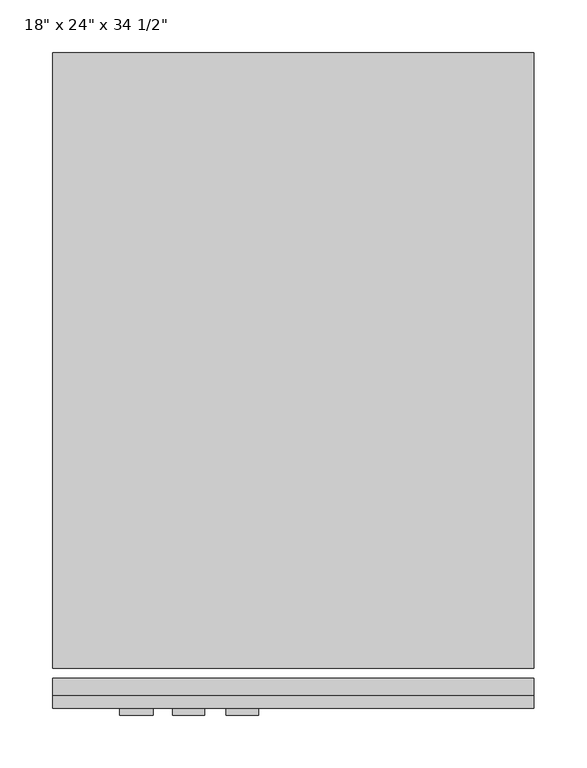
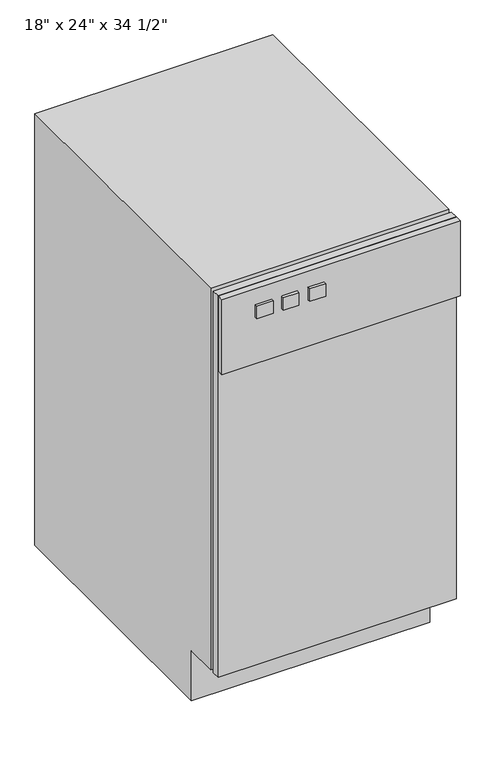
"""IFC4 building model written with IfcOpenShell, lengths in millimetres: proxy geometry."""

from ifc_helpers import new_model, si_unit, frame, origin, place, context, project, spatial, polyline, outline, extrude, source, transform, mapped, element, save


def proxy_7e1014cc(model_context):
    return source(origin(), model_context, "Body", "SweptSolid", [
        extrude(outline(polyline([(534.7174685, -38.3504352), (77.5174685, -38.3504352), (77.5174685, -22.4754352), (534.7174685, -22.4754352), (534.7174685, -38.3504352)])), frame((0.0, 0.0, 101.6), z_axis=(0.0, 0.0, 1.0), x_axis=(1.0, 0.0, 0.0)), (0.0, 0.0, 1.0), 774.7),
        extrude(outline(polyline([(534.7174685, -38.3504352), (534.7174685, -51.0504352), (77.5174685, -51.0504352), (77.5174685, -38.3504352), (534.7174685, -38.3504352)])), frame((0.0, 0.0, 723.9), z_axis=(0.0, 0.0, 1.0), x_axis=(1.0, 0.0, 0.0)), (0.0, 0.0, 1.0), 152.4),
        extrude(outline(polyline([(571.2495648, 0.0), (50.5495648, 0.0), (50.5495648, 101.6), (-12.9504352, 101.6), (-12.9504352, 876.3), (571.2495648, 876.3), (571.2495648, 0.0)])), frame((77.5174685, 0.0, 0.0), z_axis=(1.0, 0.0, 0.0), x_axis=(0.0, 1.0, 0.0)), (0.0, 0.0, 1.0), 457.2),
        extrude(outline(polyline([(172.7674685, -57.4004352), (141.0174685, -57.4004352), (141.0174685, -51.0504352), (172.7674685, -51.0504352), (172.7674685, -57.4004352)])), frame((0.0, 0.0, 818.6415009), z_axis=(0.0, 0.0, 1.0), x_axis=(1.0, 0.0, 0.0)), (0.0, 0.0, 1.0), 25.4),
        extrude(outline(polyline([(221.6847918, -57.4004352), (191.3389562, -57.4004352), (191.3389562, -51.0504352), (221.6847918, -51.0504352), (221.6847918, -57.4004352)])), frame((0.0, 0.0, 818.6415009), z_axis=(0.0, 0.0, 1.0), x_axis=(1.0, 0.0, 0.0)), (0.0, 0.0, 1.0), 25.4),
        extrude(outline(polyline([(272.969254, -57.4004352), (242.3199601, -57.4004352), (242.3199601, -51.0504352), (272.969254, -51.0504352), (272.969254, -57.4004352)])), frame((0.0, 0.0, 818.6415009), z_axis=(0.0, 0.0, 1.0), x_axis=(1.0, 0.0, 0.0)), (0.0, 0.0, 1.0), 25.4),
    ])


if __name__ == "__main__":
    model = new_model("IFC4")
    model_context = context("Model", 3, world=origin())
    ifc_project = project(units=[si_unit("LENGTHUNIT", "METRE", prefix="MILLI")], contexts=[model_context])
    site = spatial("IfcSite", under=ifc_project)
    building = spatial("IfcBuilding", under=site)
    placement = place(None, origin())
    proxy_shape = proxy_7e1014cc(model_context)
    element("IfcBuildingElementProxy", 1, Name="18\" x 24\" x 34 1/2\"", ObjectType="18\" x 24\" x 34 1/2\"", at=placement, inside=building, context=model_context, shape_type="MappedRepresentation", body=[
        mapped(proxy_shape, transform((0.0, 0.0, 0.0), x_axis=(1.0, 0.0, 0.0), y_axis=(0.0, 1.0, 0.0), z_axis=(0.0, 0.0, 1.0))),
    ])
    save(model, "model.ifc")

# Revit data of these elements
# Type "18\" x 24\" x 34 1/2\""
#   Label = "T"
#   Assembly Code = "E1090400"
#   Depth = 2' - 0"
#   Height = 2' - 10 1/2"
#   Width = 1' - 6"
#   Panel Face Material = Plastic, Opaque Black
#   Trach Compact. Material = Steel, Paint Finish, Ivory, Matte
#   Default Elevation = 0
# Element 1 (IfcBuildingElementProxy, "18\" x 24\" x 34 1/2\"")
#   Materials on its faces: "Steel, Paint Finish, Ivory, Matte", "Plastic, Opaque Black"
# Materials
#   "Plastic, Opaque Black": class "Plastic", colour RGB 0 0 0, transparency 0.05, Description = "Plastic, generic, opaque black", Cost = 0
#   "Steel, Paint Finish, Ivory, Matte": class "Metal", colour RGB 247 247 239, transparency 0, Description = "Steel, paint finish, ivory, matte", Cost = 0
